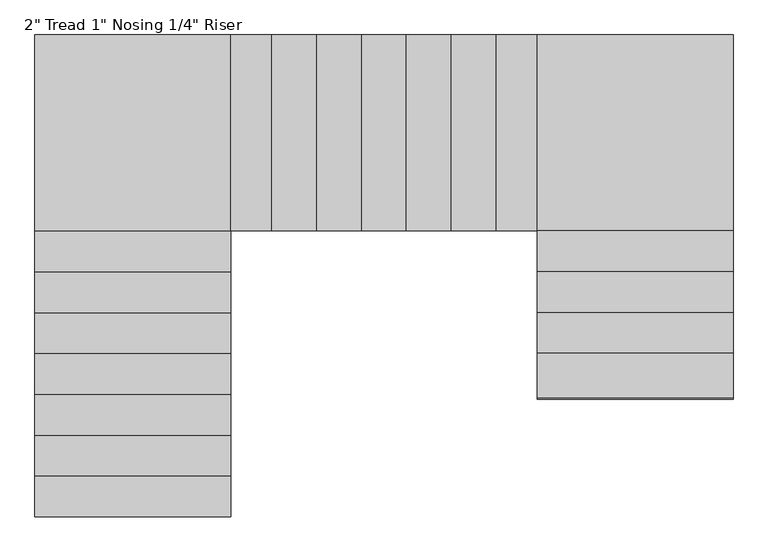
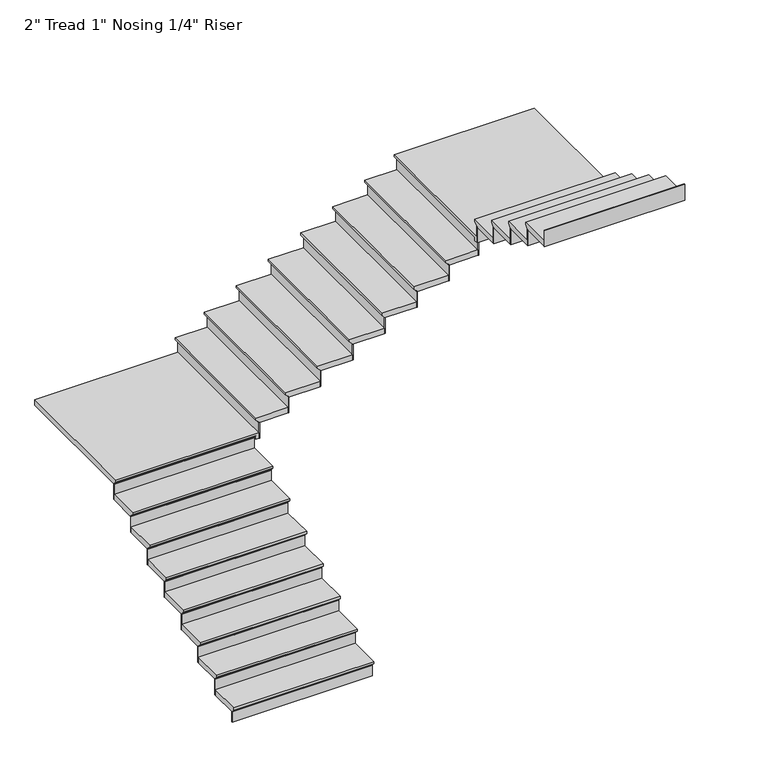
"""IFC4 building model written with IfcOpenShell, lengths in millimetres: stair flight geometry."""

from ifc_helpers import new_model, si_unit, origin, place, context, project, spatial, faceted_brep, source, transform, mapped, element, save


def stair_flight_c0b809fc(model_context):
    return source(origin(), model_context, "Body", "Brep", [
        faceted_brep([(-39731.7146233, 12415.3624892, 126.0928571), (-39731.7146233, 12415.3624892, 145.1428571), (-40950.9146233, 12415.3624892, 145.1428571), (-40950.9146233, 12415.3624892, 126.0928571), (-39731.7146233, 12440.7624892, 100.6928571), (-40950.9146233, 12440.7624892, 100.6928571), (-39731.7146233, 12694.7624892, 145.1428571), (-40950.9146233, 12694.7624892, 145.1428571), (-40950.9146233, 12440.7624892, 94.3428571), (-40950.9146233, 12694.7624892, 94.3428571), (-39731.7146233, 12694.7624892, 94.3428571), (-39731.7146233, 12440.7624892, 94.3428571)], [[[0, 1, 2, 3]], [[4, 0, 3, 5]], [[2, 1, 6, 7]], [[8, 9, 10, 11]], [[2, 7, 9, 8, 5, 3]], [[8, 11, 4, 5]], [[6, 1, 0, 4, 11, 10]], [[7, 6, 10, 9]]]),
        faceted_brep([(-39731.7146233, 12440.7624892, 94.3428571), (-39731.7146233, 12440.7624892, 0.0), (-39731.7146233, 12447.1124892, 0.0), (-39731.7146233, 12447.1124892, 94.3428571), (-40950.9146233, 12440.7624892, 94.3428571), (-40950.9146233, 12447.1124892, 94.3428571), (-40950.9146233, 12447.1124892, 0.0), (-40950.9146233, 12440.7624892, 0.0)], [[[0, 1, 2, 3]], [[4, 5, 6, 7]], [[1, 0, 4, 7]], [[2, 1, 7, 6]], [[3, 2, 6, 5]], [[0, 3, 5, 4]]]),
        faceted_brep([(-39731.7146233, 12694.7624892, 239.4857143), (-39731.7146233, 12694.7624892, 94.3428571), (-39731.7146233, 12701.1124892, 94.3428571), (-39731.7146233, 12701.1124892, 239.4857143), (-40950.9146233, 12694.7624892, 239.4857143), (-40950.9146233, 12701.1124892, 239.4857143), (-40950.9146233, 12701.1124892, 94.3428571), (-40950.9146233, 12694.7624892, 94.3428571)], [[[0, 1, 2, 3]], [[4, 5, 6, 7]], [[1, 0, 4, 7]], [[2, 1, 7, 6]], [[3, 2, 6, 5]], [[0, 3, 5, 4]]]),
        faceted_brep([(-40950.9146233, 12669.3624892, 290.2857143), (-39731.7146233, 12669.3624892, 290.2857143), (-39731.7146233, 12948.7624892, 290.2857143), (-40950.9146233, 12948.7624892, 290.2857143), (-40950.9146233, 12694.7624892, 239.4857143), (-40950.9146233, 12948.7624892, 239.4857143), (-39731.7146233, 12948.7624892, 239.4857143), (-39731.7146233, 12694.7624892, 239.4857143), (-40950.9146233, 12694.7624892, 245.8357143), (-40950.9146233, 12669.3624892, 271.2357143), (-39731.7146233, 12694.7624892, 245.8357143), (-39731.7146233, 12669.3624892, 271.2357143)], [[[0, 1, 2, 3]], [[4, 5, 6, 7]], [[0, 3, 5, 4, 8, 9]], [[4, 7, 10, 8]], [[2, 1, 11, 10, 7, 6]], [[3, 2, 6, 5]], [[11, 1, 0, 9]], [[10, 11, 9, 8]]]),
        faceted_brep([(-39731.7146233, 12948.7624892, 384.6285714), (-39731.7146233, 12948.7624892, 239.4857143), (-39731.7146233, 12955.1124892, 239.4857143), (-39731.7146233, 12955.1124892, 384.6285714), (-40950.9146233, 12948.7624892, 384.6285714), (-40950.9146233, 12955.1124892, 384.6285714), (-40950.9146233, 12955.1124892, 239.4857143), (-40950.9146233, 12948.7624892, 239.4857143)], [[[0, 1, 2, 3]], [[4, 5, 6, 7]], [[1, 0, 4, 7]], [[2, 1, 7, 6]], [[3, 2, 6, 5]], [[0, 3, 5, 4]]]),
        faceted_brep([(-40950.9146233, 12923.3624892, 435.4285714), (-39731.7146233, 12923.3624892, 435.4285714), (-39731.7146233, 13202.7624892, 435.4285714), (-40950.9146233, 13202.7624892, 435.4285714), (-40950.9146233, 12948.7624892, 384.6285714), (-40950.9146233, 13202.7624892, 384.6285714), (-39731.7146233, 13202.7624892, 384.6285714), (-39731.7146233, 12948.7624892, 384.6285714), (-40950.9146233, 12948.7624892, 390.9785714), (-40950.9146233, 12923.3624892, 416.3785714), (-39731.7146233, 12948.7624892, 390.9785714), (-39731.7146233, 12923.3624892, 416.3785714)], [[[0, 1, 2, 3]], [[4, 5, 6, 7]], [[0, 3, 5, 4, 8, 9]], [[4, 7, 10, 8]], [[2, 1, 11, 10, 7, 6]], [[3, 2, 6, 5]], [[11, 1, 0, 9]], [[10, 11, 9, 8]]]),
        faceted_brep([(-39731.7146233, 13202.7624892, 529.7714286), (-39731.7146233, 13202.7624892, 384.6285714), (-39731.7146233, 13209.1124892, 384.6285714), (-39731.7146233, 13209.1124892, 529.7714286), (-40950.9146233, 13202.7624892, 529.7714286), (-40950.9146233, 13209.1124892, 529.7714286), (-40950.9146233, 13209.1124892, 384.6285714), (-40950.9146233, 13202.7624892, 384.6285714)], [[[0, 1, 2, 3]], [[4, 5, 6, 7]], [[1, 0, 4, 7]], [[2, 1, 7, 6]], [[3, 2, 6, 5]], [[0, 3, 5, 4]]]),
        faceted_brep([(-40950.9146233, 13177.3624892, 580.5714286), (-39731.7146233, 13177.3624892, 580.5714286), (-39731.7146233, 13456.7624892, 580.5714286), (-40950.9146233, 13456.7624892, 580.5714286), (-40950.9146233, 13202.7624892, 529.7714286), (-40950.9146233, 13456.7624892, 529.7714286), (-39731.7146233, 13456.7624892, 529.7714286), (-39731.7146233, 13202.7624892, 529.7714286), (-40950.9146233, 13202.7624892, 536.1214286), (-40950.9146233, 13177.3624892, 561.5214286), (-39731.7146233, 13202.7624892, 536.1214286), (-39731.7146233, 13177.3624892, 561.5214286)], [[[0, 1, 2, 3]], [[4, 5, 6, 7]], [[0, 3, 5, 4, 8, 9]], [[4, 7, 10, 8]], [[2, 1, 11, 10, 7, 6]], [[3, 2, 6, 5]], [[11, 1, 0, 9]], [[10, 11, 9, 8]]]),
        faceted_brep([(-39731.7146233, 13456.7624892, 674.9142857), (-39731.7146233, 13456.7624892, 529.7714286), (-39731.7146233, 13463.1124892, 529.7714286), (-39731.7146233, 13463.1124892, 674.9142857), (-40950.9146233, 13456.7624892, 674.9142857), (-40950.9146233, 13463.1124892, 674.9142857), (-40950.9146233, 13463.1124892, 529.7714286), (-40950.9146233, 13456.7624892, 529.7714286)], [[[0, 1, 2, 3]], [[4, 5, 6, 7]], [[1, 0, 4, 7]], [[2, 1, 7, 6]], [[3, 2, 6, 5]], [[0, 3, 5, 4]]]),
        faceted_brep([(-40950.9146233, 13431.3624892, 725.7142857), (-39731.7146233, 13431.3624892, 725.7142857), (-39731.7146233, 13710.7624892, 725.7142857), (-40950.9146233, 13710.7624892, 725.7142857), (-40950.9146233, 13456.7624892, 674.9142857), (-40950.9146233, 13710.7624892, 674.9142857), (-39731.7146233, 13710.7624892, 674.9142857), (-39731.7146233, 13456.7624892, 674.9142857), (-40950.9146233, 13456.7624892, 681.2642857), (-40950.9146233, 13431.3624892, 706.6642857), (-39731.7146233, 13456.7624892, 681.2642857), (-39731.7146233, 13431.3624892, 706.6642857)], [[[0, 1, 2, 3]], [[4, 5, 6, 7]], [[0, 3, 5, 4, 8, 9]], [[4, 7, 10, 8]], [[2, 1, 11, 10, 7, 6]], [[3, 2, 6, 5]], [[11, 1, 0, 9]], [[10, 11, 9, 8]]]),
        faceted_brep([(-39731.7146233, 13710.7624892, 820.0571429), (-39731.7146233, 13710.7624892, 674.9142857), (-39731.7146233, 13717.1124892, 674.9142857), (-39731.7146233, 13717.1124892, 820.0571429), (-40950.9146233, 13710.7624892, 820.0571429), (-40950.9146233, 13717.1124892, 820.0571429), (-40950.9146233, 13717.1124892, 674.9142857), (-40950.9146233, 13710.7624892, 674.9142857)], [[[0, 1, 2, 3]], [[4, 5, 6, 7]], [[1, 0, 4, 7]], [[2, 1, 7, 6]], [[3, 2, 6, 5]], [[0, 3, 5, 4]]]),
        faceted_brep([(-40950.9146233, 13685.3624892, 870.8571429), (-39731.7146233, 13685.3624892, 870.8571429), (-39731.7146233, 13964.7624892, 870.8571429), (-40950.9146233, 13964.7624892, 870.8571429), (-40950.9146233, 13710.7624892, 820.0571429), (-40950.9146233, 13964.7624892, 820.0571429), (-39731.7146233, 13964.7624892, 820.0571429), (-39731.7146233, 13710.7624892, 820.0571429), (-40950.9146233, 13710.7624892, 826.4071429), (-40950.9146233, 13685.3624892, 851.8071429), (-39731.7146233, 13710.7624892, 826.4071429), (-39731.7146233, 13685.3624892, 851.8071429)], [[[0, 1, 2, 3]], [[4, 5, 6, 7]], [[0, 3, 5, 4, 8, 9]], [[4, 7, 10, 8]], [[2, 1, 11, 10, 7, 6]], [[3, 2, 6, 5]], [[11, 1, 0, 9]], [[10, 11, 9, 8]]]),
        faceted_brep([(-39731.7146233, 13964.7624892, 965.2), (-39731.7146233, 13964.7624892, 820.0571429), (-39731.7146233, 13971.1124892, 820.0571429), (-39731.7146233, 13971.1124892, 965.2), (-40950.9146233, 13964.7624892, 965.2), (-40950.9146233, 13971.1124892, 965.2), (-40950.9146233, 13971.1124892, 820.0571429), (-40950.9146233, 13964.7624892, 820.0571429)], [[[0, 1, 2, 3]], [[4, 5, 6, 7]], [[1, 0, 4, 7]], [[2, 1, 7, 6]], [[3, 2, 6, 5]], [[0, 3, 5, 4]]]),
        faceted_brep([(-40950.9146233, 13939.3624892, 1016.0), (-39731.7146233, 13939.3624892, 1016.0), (-39731.7146233, 14218.7624892, 1016.0), (-40950.9146233, 14218.7624892, 1016.0), (-40950.9146233, 13964.7624892, 965.2), (-40950.9146233, 14218.7624892, 965.2), (-39731.7146233, 14218.7624892, 965.2), (-39731.7146233, 13964.7624892, 965.2), (-40950.9146233, 13964.7624892, 971.55), (-40950.9146233, 13939.3624892, 996.95), (-39731.7146233, 13964.7624892, 971.55), (-39731.7146233, 13939.3624892, 996.95)], [[[0, 1, 2, 3]], [[4, 5, 6, 7]], [[0, 3, 5, 4, 8, 9]], [[4, 7, 10, 8]], [[2, 1, 11, 10, 7, 6]], [[3, 2, 6, 5]], [[11, 1, 0, 9]], [[10, 11, 9, 8]]]),
        faceted_brep([(-39731.7146233, 14218.7624892, 1110.3428571), (-39731.7146233, 14218.7624892, 965.2), (-39731.7146233, 14225.1124892, 965.2), (-39731.7146233, 14225.1124892, 1110.3428571), (-40950.9146233, 14218.7624892, 1110.3428571), (-40950.9146233, 14225.1124892, 1110.3428571), (-40950.9146233, 14225.1124892, 965.2), (-40950.9146233, 14218.7624892, 965.2)], [[[0, 1, 2, 3]], [[4, 5, 6, 7]], [[1, 0, 4, 7]], [[2, 1, 7, 6]], [[3, 2, 6, 5]], [[0, 3, 5, 4]]]),
        faceted_brep([(-39706.3146233, 15412.5624892, 1161.1428571), (-40950.9146233, 15412.5624892, 1161.1428571), (-40950.9146233, 14193.3624892, 1161.1428571), (-39706.3146233, 14193.3624892, 1161.1428571), (-40950.9146233, 15412.5624892, 1110.3428571), (-39706.3146233, 15412.5624892, 1110.3428571), (-39706.3146233, 14193.3624892, 1110.3428571), (-39731.7146233, 14193.3624892, 1110.3428571), (-39731.7146233, 14218.7624892, 1110.3428571), (-40950.9146233, 14218.7624892, 1110.3428571), (-40950.9146233, 14218.7624892, 1116.6928571), (-40950.9146233, 14193.3624892, 1142.0928571), (-39731.7146233, 14218.7624892, 1116.6928571), (-39731.7146233, 14193.3624892, 1142.0928571)], [[[0, 1, 2, 3]], [[4, 5, 6, 7, 8, 9]], [[1, 0, 5, 4]], [[2, 1, 4, 9, 10, 11]], [[9, 8, 12, 10]], [[8, 7, 13, 12]], [[3, 2, 11, 13, 7, 6]], [[0, 3, 6, 5]], [[11, 10, 12, 13]]]),
        faceted_brep([(-39706.3146233, 14193.3624892, 1255.4857143), (-39706.3146233, 14193.3624892, 1110.3428571), (-39699.9646233, 14193.3624892, 1110.3428571), (-39699.9646233, 14193.3624892, 1255.4857143), (-39706.3146233, 15412.5624892, 1255.4857143), (-39699.9646233, 15412.5624892, 1255.4857143), (-39699.9646233, 15412.5624892, 1110.3428571), (-39706.3146233, 15412.5624892, 1110.3428571)], [[[0, 1, 2, 3]], [[4, 5, 6, 7]], [[1, 0, 4, 7]], [[2, 1, 7, 6]], [[3, 2, 6, 5]], [[0, 3, 5, 4]]]),
        faceted_brep([(-39731.7146233, 15412.5624892, 1306.2857143), (-39731.7146233, 14193.3624892, 1306.2857143), (-39452.3146233, 14193.3624892, 1306.2857143), (-39452.3146233, 15412.5624892, 1306.2857143), (-39706.3146233, 15412.5624892, 1255.4857143), (-39452.3146233, 15412.5624892, 1255.4857143), (-39452.3146233, 14193.3624892, 1255.4857143), (-39706.3146233, 14193.3624892, 1255.4857143), (-39706.3146233, 15412.5624892, 1261.8357143), (-39731.7146233, 15412.5624892, 1287.2357143), (-39706.3146233, 14193.3624892, 1261.8357143), (-39731.7146233, 14193.3624892, 1287.2357143)], [[[0, 1, 2, 3]], [[4, 5, 6, 7]], [[0, 3, 5, 4, 8, 9]], [[4, 7, 10, 8]], [[2, 1, 11, 10, 7, 6]], [[3, 2, 6, 5]], [[11, 1, 0, 9]], [[10, 11, 9, 8]]]),
        faceted_brep([(-39452.3146233, 14193.3624892, 1400.6285714), (-39452.3146233, 14193.3624892, 1255.4857143), (-39445.9646233, 14193.3624892, 1255.4857143), (-39445.9646233, 14193.3624892, 1400.6285714), (-39452.3146233, 15412.5624892, 1400.6285714), (-39445.9646233, 15412.5624892, 1400.6285714), (-39445.9646233, 15412.5624892, 1255.4857143), (-39452.3146233, 15412.5624892, 1255.4857143)], [[[0, 1, 2, 3]], [[4, 5, 6, 7]], [[1, 0, 4, 7]], [[2, 1, 7, 6]], [[3, 2, 6, 5]], [[0, 3, 5, 4]]]),
        faceted_brep([(-39477.7146233, 15412.5624892, 1451.4285714), (-39477.7146233, 14193.3624892, 1451.4285714), (-39172.9146233, 14193.3624892, 1451.4285714), (-39172.9146233, 15412.5624892, 1451.4285714), (-39452.3146233, 15412.5624892, 1400.6285714), (-39172.9146233, 15412.5624892, 1400.6285714), (-39172.9146233, 14193.3624892, 1400.6285714), (-39452.3146233, 14193.3624892, 1400.6285714), (-39452.3146233, 15412.5624892, 1406.9785714), (-39477.7146233, 15412.5624892, 1432.3785714), (-39452.3146233, 14193.3624892, 1406.9785714), (-39477.7146233, 14193.3624892, 1432.3785714)], [[[0, 1, 2, 3]], [[4, 5, 6, 7]], [[0, 3, 5, 4, 8, 9]], [[4, 7, 10, 8]], [[2, 1, 11, 10, 7, 6]], [[3, 2, 6, 5]], [[11, 1, 0, 9]], [[10, 11, 9, 8]]]),
        faceted_brep([(-39172.9146233, 14193.3624892, 1545.7714286), (-39172.9146233, 14193.3624892, 1400.6285714), (-39166.5646233, 14193.3624892, 1400.6285714), (-39166.5646233, 14193.3624892, 1545.7714286), (-39172.9146233, 15412.5624892, 1545.7714286), (-39166.5646233, 15412.5624892, 1545.7714286), (-39166.5646233, 15412.5624892, 1400.6285714), (-39172.9146233, 15412.5624892, 1400.6285714)], [[[0, 1, 2, 3]], [[4, 5, 6, 7]], [[1, 0, 4, 7]], [[2, 1, 7, 6]], [[3, 2, 6, 5]], [[0, 3, 5, 4]]]),
        faceted_brep([(-39198.3146233, 15412.5624892, 1596.5714286), (-39198.3146233, 14193.3624892, 1596.5714286), (-38893.5146233, 14193.3624892, 1596.5714286), (-38893.5146233, 15412.5624892, 1596.5714286), (-39172.9146233, 15412.5624892, 1545.7714286), (-38893.5146233, 15412.5624892, 1545.7714286), (-38893.5146233, 14193.3624892, 1545.7714286), (-39172.9146233, 14193.3624892, 1545.7714286), (-39172.9146233, 15412.5624892, 1552.1214286), (-39198.3146233, 15412.5624892, 1577.5214286), (-39172.9146233, 14193.3624892, 1552.1214286), (-39198.3146233, 14193.3624892, 1577.5214286)], [[[0, 1, 2, 3]], [[4, 5, 6, 7]], [[0, 3, 5, 4, 8, 9]], [[4, 7, 10, 8]], [[2, 1, 11, 10, 7, 6]], [[3, 2, 6, 5]], [[11, 1, 0, 9]], [[10, 11, 9, 8]]]),
        faceted_brep([(-38893.5146233, 14193.3624892, 1690.9142857), (-38893.5146233, 14193.3624892, 1545.7714286), (-38887.1646233, 14193.3624892, 1545.7714286), (-38887.1646233, 14193.3624892, 1690.9142857), (-38893.5146233, 15412.5624892, 1690.9142857), (-38887.1646233, 15412.5624892, 1690.9142857), (-38887.1646233, 15412.5624892, 1545.7714286), (-38893.5146233, 15412.5624892, 1545.7714286)], [[[0, 1, 2, 3]], [[4, 5, 6, 7]], [[1, 0, 4, 7]], [[2, 1, 7, 6]], [[3, 2, 6, 5]], [[0, 3, 5, 4]]]),
        faceted_brep([(-38918.9146233, 15412.5624892, 1741.7142857), (-38918.9146233, 14193.3624892, 1741.7142857), (-38614.1146233, 14193.3624892, 1741.7142857), (-38614.1146233, 15412.5624892, 1741.7142857), (-38893.5146233, 15412.5624892, 1690.9142857), (-38614.1146233, 15412.5624892, 1690.9142857), (-38614.1146233, 14193.3624892, 1690.9142857), (-38893.5146233, 14193.3624892, 1690.9142857), (-38893.5146233, 15412.5624892, 1697.2642857), (-38918.9146233, 15412.5624892, 1722.6642857), (-38893.5146233, 14193.3624892, 1697.2642857), (-38918.9146233, 14193.3624892, 1722.6642857)], [[[0, 1, 2, 3]], [[4, 5, 6, 7]], [[0, 3, 5, 4, 8, 9]], [[4, 7, 10, 8]], [[2, 1, 11, 10, 7, 6]], [[3, 2, 6, 5]], [[11, 1, 0, 9]], [[10, 11, 9, 8]]]),
        faceted_brep([(-38614.1146233, 14193.3624892, 1836.0571429), (-38614.1146233, 14193.3624892, 1690.9142857), (-38607.7646233, 14193.3624892, 1690.9142857), (-38607.7646233, 14193.3624892, 1836.0571429), (-38614.1146233, 15412.5624892, 1836.0571429), (-38607.7646233, 15412.5624892, 1836.0571429), (-38607.7646233, 15412.5624892, 1690.9142857), (-38614.1146233, 15412.5624892, 1690.9142857)], [[[0, 1, 2, 3]], [[4, 5, 6, 7]], [[1, 0, 4, 7]], [[2, 1, 7, 6]], [[3, 2, 6, 5]], [[0, 3, 5, 4]]]),
        faceted_brep([(-38639.5146233, 15412.5624892, 1886.8571429), (-38639.5146233, 14193.3624892, 1886.8571429), (-38334.7146233, 14193.3624892, 1886.8571429), (-38334.7146233, 15412.5624892, 1886.8571429), (-38614.1146233, 15412.5624892, 1836.0571429), (-38334.7146233, 15412.5624892, 1836.0571429), (-38334.7146233, 14193.3624892, 1836.0571429), (-38614.1146233, 14193.3624892, 1836.0571429), (-38614.1146233, 15412.5624892, 1842.4071429), (-38639.5146233, 15412.5624892, 1867.8071429), (-38614.1146233, 14193.3624892, 1842.4071429), (-38639.5146233, 14193.3624892, 1867.8071429)], [[[0, 1, 2, 3]], [[4, 5, 6, 7]], [[0, 3, 5, 4, 8, 9]], [[4, 7, 10, 8]], [[2, 1, 11, 10, 7, 6]], [[3, 2, 6, 5]], [[11, 1, 0, 9]], [[10, 11, 9, 8]]]),
        faceted_brep([(-38334.7146233, 14193.3624892, 1981.2), (-38334.7146233, 14193.3624892, 1836.0571429), (-38328.3646233, 14193.3624892, 1836.0571429), (-38328.3646233, 14193.3624892, 1981.2), (-38334.7146233, 15412.5624892, 1981.2), (-38328.3646233, 15412.5624892, 1981.2), (-38328.3646233, 15412.5624892, 1836.0571429), (-38334.7146233, 15412.5624892, 1836.0571429)], [[[0, 1, 2, 3]], [[4, 5, 6, 7]], [[1, 0, 4, 7]], [[2, 1, 7, 6]], [[3, 2, 6, 5]], [[0, 3, 5, 4]]]),
        faceted_brep([(-38360.1146233, 15412.5624892, 2032.0), (-38360.1146233, 14193.3624892, 2032.0), (-38055.3146233, 14193.3624892, 2032.0), (-38055.3146233, 15412.5624892, 2032.0), (-38334.7146233, 15412.5624892, 1981.2), (-38055.3146233, 15412.5624892, 1981.2), (-38055.3146233, 14193.3624892, 1981.2), (-38334.7146233, 14193.3624892, 1981.2), (-38334.7146233, 15412.5624892, 1987.55), (-38360.1146233, 15412.5624892, 2012.95), (-38334.7146233, 14193.3624892, 1987.55), (-38360.1146233, 14193.3624892, 2012.95)], [[[0, 1, 2, 3]], [[4, 5, 6, 7]], [[0, 3, 5, 4, 8, 9]], [[4, 7, 10, 8]], [[2, 1, 11, 10, 7, 6]], [[3, 2, 6, 5]], [[11, 1, 0, 9]], [[10, 11, 9, 8]]]),
        faceted_brep([(-38055.3146233, 14193.3624892, 2126.3428571), (-38055.3146233, 14193.3624892, 1981.2), (-38048.9646233, 14193.3624892, 1981.2), (-38048.9646233, 14193.3624892, 2126.3428571), (-38055.3146233, 15412.5624892, 2126.3428571), (-38048.9646233, 15412.5624892, 2126.3428571), (-38048.9646233, 15412.5624892, 1981.2), (-38055.3146233, 15412.5624892, 1981.2)], [[[0, 1, 2, 3]], [[4, 5, 6, 7]], [[1, 0, 4, 7]], [[2, 1, 7, 6]], [[3, 2, 6, 5]], [[0, 3, 5, 4]]]),
        faceted_brep([(-38080.7146233, 15412.5624892, 2177.1428571), (-38080.7146233, 14193.3624892, 2177.1428571), (-37801.3146233, 14193.3624892, 2177.1428571), (-37801.3146233, 15412.5624892, 2177.1428571), (-38055.3146233, 15412.5624892, 2126.3428571), (-37801.3146233, 15412.5624892, 2126.3428571), (-37801.3146233, 14193.3624892, 2126.3428571), (-38055.3146233, 14193.3624892, 2126.3428571), (-38055.3146233, 15412.5624892, 2132.6928571), (-38080.7146233, 15412.5624892, 2158.0928571), (-38055.3146233, 14193.3624892, 2132.6928571), (-38080.7146233, 14193.3624892, 2158.0928571)], [[[0, 1, 2, 3]], [[4, 5, 6, 7]], [[0, 3, 5, 4, 8, 9]], [[4, 7, 10, 8]], [[2, 1, 11, 10, 7, 6]], [[3, 2, 6, 5]], [[11, 1, 0, 9]], [[10, 11, 9, 8]]]),
        faceted_brep([(-37801.3146233, 14193.3624892, 2271.4857143), (-37801.3146233, 14193.3624892, 2126.3428571), (-37794.9646233, 14193.3624892, 2126.3428571), (-37794.9646233, 14193.3624892, 2271.4857143), (-37801.3146233, 15412.5624892, 2271.4857143), (-37794.9646233, 15412.5624892, 2271.4857143), (-37794.9646233, 15412.5624892, 2126.3428571), (-37801.3146233, 15412.5624892, 2126.3428571)], [[[0, 1, 2, 3]], [[4, 5, 6, 7]], [[1, 0, 4, 7]], [[2, 1, 7, 6]], [[3, 2, 6, 5]], [[0, 3, 5, 4]]]),
        faceted_brep([(-36607.5146233, 14167.9624892, 2322.2857143), (-36607.5146233, 15412.5624892, 2322.2857143), (-37826.7146233, 15412.5624892, 2322.2857143), (-37826.7146233, 14167.9624892, 2322.2857143), (-36607.5146233, 15412.5624892, 2271.4857143), (-36607.5146233, 14167.9624892, 2271.4857143), (-37826.7146233, 14167.9624892, 2271.4857143), (-37826.7146233, 14193.3624892, 2271.4857143), (-37801.3146233, 14193.3624892, 2271.4857143), (-37801.3146233, 15412.5624892, 2271.4857143), (-37801.3146233, 15412.5624892, 2277.8357143), (-37826.7146233, 15412.5624892, 2303.2357143), (-37801.3146233, 14193.3624892, 2277.8357143), (-37826.7146233, 14193.3624892, 2303.2357143)], [[[0, 1, 2, 3]], [[4, 5, 6, 7, 8, 9]], [[1, 0, 5, 4]], [[2, 1, 4, 9, 10, 11]], [[9, 8, 12, 10]], [[8, 7, 13, 12]], [[3, 2, 11, 13, 7, 6]], [[0, 3, 6, 5]], [[11, 10, 12, 13]]]),
        faceted_brep([(-37826.7146233, 14167.9624892, 2416.6285714), (-37826.7146233, 14167.9624892, 2271.4857143), (-37826.7146233, 14161.6124892, 2271.4857143), (-37826.7146233, 14161.6124892, 2416.6285714), (-36607.5146233, 14167.9624892, 2416.6285714), (-36607.5146233, 14161.6124892, 2416.6285714), (-36607.5146233, 14161.6124892, 2271.4857143), (-36607.5146233, 14167.9624892, 2271.4857143)], [[[0, 1, 2, 3]], [[4, 5, 6, 7]], [[1, 0, 4, 7]], [[2, 1, 7, 6]], [[3, 2, 6, 5]], [[0, 3, 5, 4]]]),
        faceted_brep([(-36607.5146233, 14193.3624892, 2467.4285714), (-37826.7146233, 14193.3624892, 2467.4285714), (-37826.7146233, 13913.9624892, 2467.4285714), (-36607.5146233, 13913.9624892, 2467.4285714), (-36607.5146233, 14167.9624892, 2416.6285714), (-36607.5146233, 13913.9624892, 2416.6285714), (-37826.7146233, 13913.9624892, 2416.6285714), (-37826.7146233, 14167.9624892, 2416.6285714), (-36607.5146233, 14167.9624892, 2422.9785714), (-36607.5146233, 14193.3624892, 2448.3785714), (-37826.7146233, 14167.9624892, 2422.9785714), (-37826.7146233, 14193.3624892, 2448.3785714)], [[[0, 1, 2, 3]], [[4, 5, 6, 7]], [[0, 3, 5, 4, 8, 9]], [[4, 7, 10, 8]], [[2, 1, 11, 10, 7, 6]], [[3, 2, 6, 5]], [[11, 1, 0, 9]], [[10, 11, 9, 8]]]),
        faceted_brep([(-37826.7146233, 13913.9624892, 2561.7714286), (-37826.7146233, 13913.9624892, 2416.6285714), (-37826.7146233, 13907.6124892, 2416.6285714), (-37826.7146233, 13907.6124892, 2561.7714286), (-36607.5146233, 13913.9624892, 2561.7714286), (-36607.5146233, 13907.6124892, 2561.7714286), (-36607.5146233, 13907.6124892, 2416.6285714), (-36607.5146233, 13913.9624892, 2416.6285714)], [[[0, 1, 2, 3]], [[4, 5, 6, 7]], [[1, 0, 4, 7]], [[2, 1, 7, 6]], [[3, 2, 6, 5]], [[0, 3, 5, 4]]]),
        faceted_brep([(-36607.5146233, 13939.3624892, 2612.5714286), (-37826.7146233, 13939.3624892, 2612.5714286), (-37826.7146233, 13659.9624892, 2612.5714286), (-36607.5146233, 13659.9624892, 2612.5714286), (-36607.5146233, 13913.9624892, 2561.7714286), (-36607.5146233, 13659.9624892, 2561.7714286), (-37826.7146233, 13659.9624892, 2561.7714286), (-37826.7146233, 13913.9624892, 2561.7714286), (-36607.5146233, 13913.9624892, 2568.1214286), (-36607.5146233, 13939.3624892, 2593.5214286), (-37826.7146233, 13913.9624892, 2568.1214286), (-37826.7146233, 13939.3624892, 2593.5214286)], [[[0, 1, 2, 3]], [[4, 5, 6, 7]], [[0, 3, 5, 4, 8, 9]], [[4, 7, 10, 8]], [[2, 1, 11, 10, 7, 6]], [[3, 2, 6, 5]], [[11, 1, 0, 9]], [[10, 11, 9, 8]]]),
        faceted_brep([(-37826.7146233, 13659.9624892, 2706.9142857), (-37826.7146233, 13659.9624892, 2561.7714286), (-37826.7146233, 13653.6124892, 2561.7714286), (-37826.7146233, 13653.6124892, 2706.9142857), (-36607.5146233, 13659.9624892, 2706.9142857), (-36607.5146233, 13653.6124892, 2706.9142857), (-36607.5146233, 13653.6124892, 2561.7714286), (-36607.5146233, 13659.9624892, 2561.7714286)], [[[0, 1, 2, 3]], [[4, 5, 6, 7]], [[1, 0, 4, 7]], [[2, 1, 7, 6]], [[3, 2, 6, 5]], [[0, 3, 5, 4]]]),
        faceted_brep([(-36607.5146233, 13685.3624892, 2757.7142857), (-37826.7146233, 13685.3624892, 2757.7142857), (-37826.7146233, 13405.9624892, 2757.7142857), (-36607.5146233, 13405.9624892, 2757.7142857), (-36607.5146233, 13659.9624892, 2706.9142857), (-36607.5146233, 13405.9624892, 2706.9142857), (-37826.7146233, 13405.9624892, 2706.9142857), (-37826.7146233, 13659.9624892, 2706.9142857), (-36607.5146233, 13659.9624892, 2713.2642857), (-36607.5146233, 13685.3624892, 2738.6642857), (-37826.7146233, 13659.9624892, 2713.2642857), (-37826.7146233, 13685.3624892, 2738.6642857)], [[[0, 1, 2, 3]], [[4, 5, 6, 7]], [[0, 3, 5, 4, 8, 9]], [[4, 7, 10, 8]], [[2, 1, 11, 10, 7, 6]], [[3, 2, 6, 5]], [[11, 1, 0, 9]], [[10, 11, 9, 8]]]),
        faceted_brep([(-37826.7146233, 13405.9624892, 2852.0571429), (-37826.7146233, 13405.9624892, 2706.9142857), (-37826.7146233, 13399.6124892, 2706.9142857), (-37826.7146233, 13399.6124892, 2852.0571429), (-36607.5146233, 13405.9624892, 2852.0571429), (-36607.5146233, 13399.6124892, 2852.0571429), (-36607.5146233, 13399.6124892, 2706.9142857), (-36607.5146233, 13405.9624892, 2706.9142857)], [[[0, 1, 2, 3]], [[4, 5, 6, 7]], [[1, 0, 4, 7]], [[2, 1, 7, 6]], [[3, 2, 6, 5]], [[0, 3, 5, 4]]]),
        faceted_brep([(-37826.7146233, 13151.9624892, 2997.2), (-37826.7146233, 13151.9624892, 2852.0571429), (-37826.7146233, 13145.6124892, 2852.0571429), (-37826.7146233, 13145.6124892, 2997.2), (-36607.5146233, 13151.9624892, 2997.2), (-36607.5146233, 13145.6124892, 2997.2), (-36607.5146233, 13145.6124892, 2852.0571429), (-36607.5146233, 13151.9624892, 2852.0571429)], [[[0, 1, 2, 3]], [[4, 5, 6, 7]], [[1, 0, 4, 7]], [[2, 1, 7, 6]], [[3, 2, 6, 5]], [[0, 3, 5, 4]]]),
        faceted_brep([(-36607.5146233, 13431.3624892, 2902.8571429), (-37826.7146233, 13431.3624892, 2902.8571429), (-37826.7146233, 13151.9624892, 2902.8571429), (-36607.5146233, 13151.9624892, 2902.8571429), (-36607.5146233, 13405.9624892, 2852.0571429), (-36607.5146233, 13151.9624892, 2852.0571429), (-37826.7146233, 13151.9624892, 2852.0571429), (-37826.7146233, 13405.9624892, 2852.0571429), (-36607.5146233, 13405.9624892, 2858.4071429), (-36607.5146233, 13431.3624892, 2883.8071429), (-37826.7146233, 13405.9624892, 2858.4071429), (-37826.7146233, 13431.3624892, 2883.8071429)], [[[0, 1, 2, 3]], [[4, 5, 6, 7]], [[0, 3, 5, 4, 8, 9]], [[4, 7, 10, 8]], [[2, 1, 11, 10, 7, 6]], [[3, 2, 6, 5]], [[11, 1, 0, 9]], [[10, 11, 9, 8]]]),
    ])


if __name__ == "__main__":
    model = new_model("IFC4")
    model_context = context("Model", 3, world=origin())
    ifc_project = project(units=[si_unit("LENGTHUNIT", "METRE", prefix="MILLI")], contexts=[model_context])
    site = spatial("IfcSite", under=ifc_project)
    building = spatial("IfcBuilding", under=site)
    placement = place(None, origin())
    stair_flight_shape = stair_flight_c0b809fc(model_context)
    element("IfcStairFlight", 1, ObjectType="2\" Tread 1\" Nosing 1/4\" Riser", at=placement, inside=building, context=model_context, shape_type="MappedRepresentation", body=[
        mapped(stair_flight_shape, transform((0.0, 0.0, 0.0), x_axis=(1.0, 0.0, 0.0), y_axis=(0.0, 1.0, 0.0), z_axis=(0.0, 0.0, 1.0))),
    ])
    save(model, "model.ifc")
